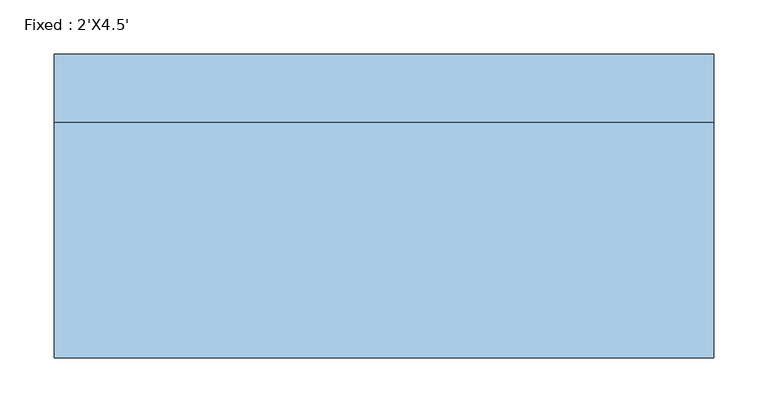
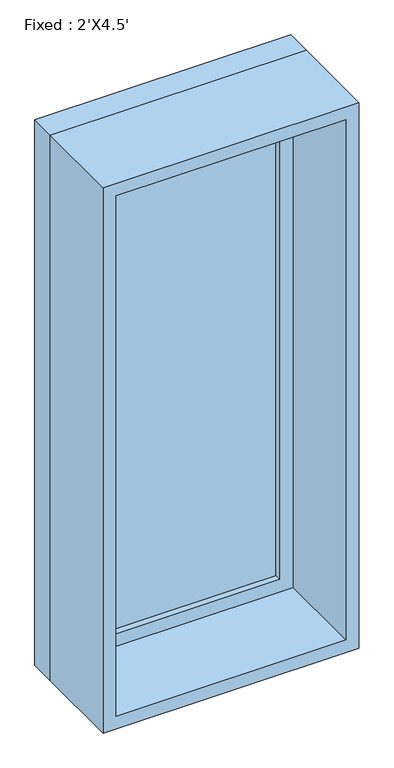
"""IFC4 building model written with IfcOpenShell, lengths in millimetres: window geometry, Fixed : 2'X4.5'."""

from ifc_helpers import new_model, si_unit, frame, origin, place, context, project, spatial, polyline, outline, extrude, source, transform, mapped, element, save


def fixed_2_x4_5_07468de1(model_context):
    return source(origin(), model_context, "Body", "SweptSolid", [
        extrude(outline(polyline([(203.2, 92.775), (-279.4, 92.775), (-279.4, 105.475), (203.2, 105.475), (203.2, 92.775)])), frame((0.0, 0.0, 825.5), z_axis=(0.0, 0.0, 1.0), x_axis=(1.0, 0.0, 0.0)), (0.0, 0.0, 1.0), 1244.6),
        extrude(outline(polyline([(2114.55, -323.85), (781.05, -323.85), (781.05, 247.65), (2114.55, 247.65), (2114.55, -323.85)]), holes=[polyline([(2070.1, -279.4), (2070.1, 203.2), (825.5, 203.2), (825.5, -279.4), (2070.1, -279.4)])]), frame((0.0, 76.9, 0.0), z_axis=(0.0, 1.0, 0.0), x_axis=(0.0, 0.0, 1.0)), (0.0, 0.0, 1.0), 44.45),
        extrude(outline(polyline([(2133.6, -342.9), (762.0, -342.9), (762.0, 266.7), (2133.6, 266.7), (2133.6, -342.9)]), holes=[polyline([(2101.85, -311.15), (2101.85, 234.95), (793.75, 234.95), (793.75, -311.15), (2101.85, -311.15)])]), frame((0.0, -140.4, 0.0), z_axis=(0.0, 1.0, 0.0), x_axis=(0.0, 0.0, 1.0)), (0.0, 0.0, 1.0), 217.3),
        extrude(outline(polyline([(2133.6, 266.7), (2133.6, -342.9), (762.0, -342.9), (762.0, 266.7), (2133.6, 266.7)]), holes=[polyline([(2114.55, 247.65), (781.05, 247.65), (781.05, -323.85), (2114.55, -323.85), (2114.55, 247.65)])]), frame((0.0, 76.9, 0.0), z_axis=(0.0, 1.0, 0.0), x_axis=(0.0, 0.0, 1.0)), (0.0, 0.0, 1.0), 63.5),
    ])


if __name__ == "__main__":
    model = new_model("IFC4")
    model_context = context("Model", 3, world=origin())
    ifc_project = project(units=[si_unit("LENGTHUNIT", "METRE", prefix="MILLI")], contexts=[model_context])
    site = spatial("IfcSite", under=ifc_project)
    building = spatial("IfcBuilding", under=site)
    placement = place(None, origin())
    fixed_2_x4_5_shape = fixed_2_x4_5_07468de1(model_context)
    element("IfcWindow", 1, ObjectType="Fixed : 2'X4.5'", at=placement, inside=building, context=model_context, shape_type="MappedRepresentation", body=[
        mapped(fixed_2_x4_5_shape, transform((0.0, 0.0, 0.0), x_axis=(1.0, 0.0, 0.0), y_axis=(0.0, 1.0, 0.0), z_axis=(0.0, 0.0, 1.0))),
    ])
    save(model, "model.ifc")

# Revit data of these elements
# Type "Fixed : 2'X4.5'"
#   Type Mark = "12"
#   Assembly Code = "B2020100"
#   Height = 4' - 6"
#   Default Sill Height = 2' - 6"
#   Width = 2' - 0"
#   Window Inset = 0' - 0 3/4"
#   Glass Pane Material = Glass
#   Sash Material = Sash
#   Wall Closure = (empty or 0)
# Element 1 (IfcWindow, "Fixed : 2'X4.5'")
#   Materials on its faces: "Sash", "Glass"
# Materials
#   "Glass": class "Glass", colour RGB 218 227 224, transparency 0.85, Description = "Soda Lime Glass", Cost = 0
#   "Sash": class "Wood", colour RGB 136 99 55, transparency 0
